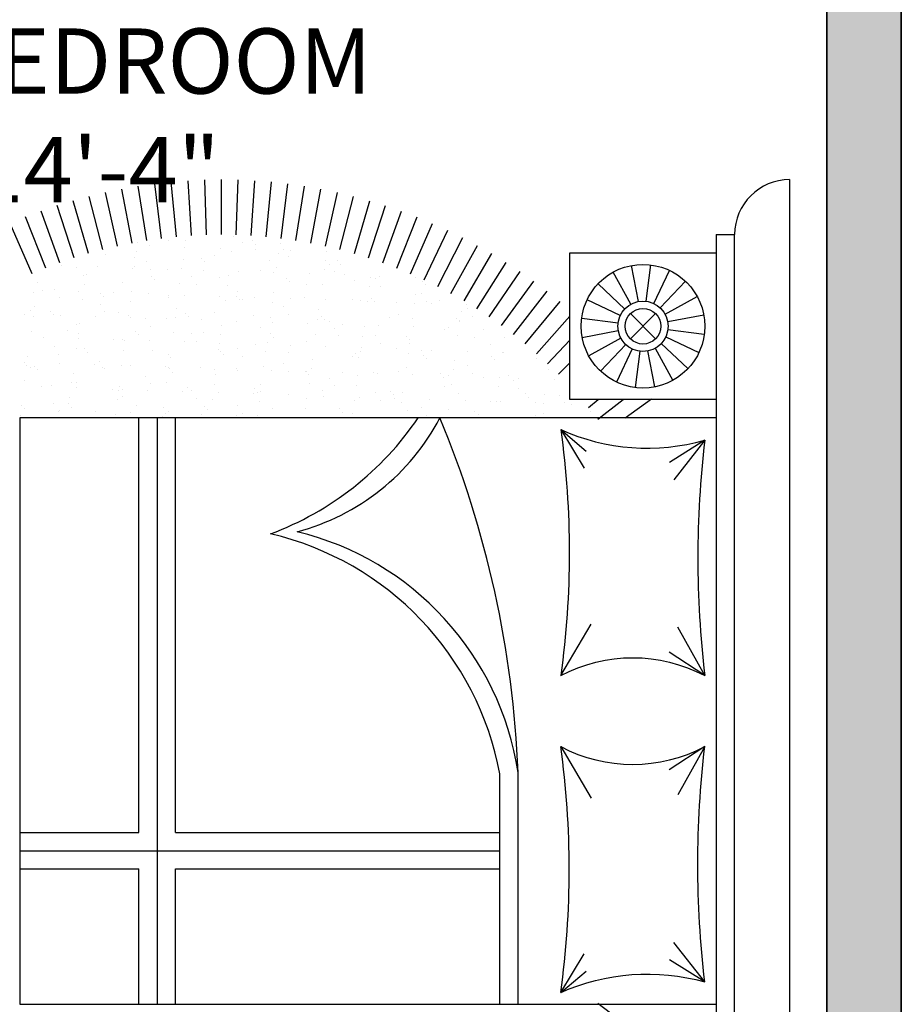
# Model space of a CAD drawing. Units: inches. Extents: x 1566 to 2546, y 1087 to 2705.
# Tile 17 of 27: x 2364 to 2458, y 1243 to 1349. Entities that reach past the tile are written whole.
import ezdxf

# ---------------------------------------------------------------- set-up
doc = ezdxf.new("R2010")
doc.units = ezdxf.units.IN
for name, color, linetype, lineweight in [('A-AREA-IDEN', 7, 'Continuous', 18), ('A-FURN', 8, 'Continuous', 18), ('A-WALL', 7, 'Continuous', 35), ('A-WALL-PATT', 8, 'Continuous', 13)]:
    doc.layers.add(name, color=color, linetype=linetype, lineweight=lineweight)
for name, color, linetype in [('A-FRN', 11, 'Continuous'), ('A-HT', 15, 'Continuous'), ('L-HT', 1, 'Continuous')]:
    doc.layers.add(name, color=color, linetype=linetype)
doc.styles.get("Standard").update_dxf_attribs({"font": 'arial.ttf'})

# ---------------------------------------------------------------- blocks, each defined once
blk = doc.blocks.new('*X21')
at = {"color": 0}
for p, q in [((1.1667, 2.0955), (1.1667, 2.0955)), ((1.1927, 2.0989), (1.1927, 2.0989)), ((0.9061, 2.0695), (0.9061, 2.0695)), ((0.9169, 2.0861), (0.9169, 2.0861)), ((0.9642, 2.0688), (0.9642, 2.0688)), ((1.0321, 2.0777), (1.0321, 2.0777)), ((1.0477, 2.0878), (1.0477, 2.0878)), ((1.0582, 2.0812), (1.0582, 2.0812)), ((1.0618, 2.0698), (1.0618, 2.0698)), ((1.0988, 2.0865), (1.0988, 2.0865)), ((1.1756, 2.0872), (1.1756, 2.0872)), ((0.8296, 2.0511), (0.8296, 2.0511)), ((0.8589, 2.0624), (0.8589, 2.0624)), ((0.8975, 2.06), (0.8975, 2.06)), ((0.9236, 2.0635), (0.9236, 2.0635)), ((1.059, 2.0607), (1.059, 2.0607)), ((1.0682, 2.0523), (1.0682, 2.0523)), ((0.8524, 2.0367), (0.8524, 2.0367)), ((0.9087, 2.0168), (0.9087, 2.0168)), ((0.9803, 2.0361), (0.9803, 2.0361)), ((1.1153, 2.0409), (1.1153, 2.0409)), ((0.8495, 2.0061), (0.8495, 2.0061)), ((0.8706, 1.9927), (0.8706, 1.9927)), ((0.9179, 2.0084), (0.9179, 2.0084)), ((0.92, 1.9898), (0.92, 1.9898)), ((1.0052, 2.0064), (1.0052, 2.0064)), ((1.0263, 1.993), (1.0263, 1.993)), ((1.0509, 1.9915), (1.0509, 1.9915)), ((1.1117, 2.0124), (1.1117, 2.0124)), ((1.1609, 2.0067), (1.1609, 2.0067)), ((1.1788, 1.9909), (1.1788, 1.9909)), ((1.182, 1.9932), (1.182, 1.9932)), ((0.785, 1.9849), (0.785, 1.9849)), ((0.9614, 1.9685), (0.9614, 1.9685)), ((1.1449, 1.9631), (1.1449, 1.9631)), ((1.1614, 1.9668), (1.1614, 1.9668)), ((0.7908, 1.944), (0.7908, 1.944)), ((0.8555, 1.9403), (0.8555, 1.9403)), ((0.9436, 1.9366), (0.9436, 1.9366)), ((0.9465, 1.9443), (0.9465, 1.9443)), ((0.9697, 1.9401), (0.9697, 1.9401)), ((0.9834, 1.9397), (0.9834, 1.9397)), ((1.0103, 1.9454), (1.0103, 1.9454)), ((1.0782, 1.9544), (1.0782, 1.9544)), ((1.1022, 1.9446), (1.1022, 1.9446)), ((1.1043, 1.9578), (1.1043, 1.9578)), ((1.1185, 1.9446), (1.1185, 1.9446)), ((1.1707, 1.9584), (1.1707, 1.9584)), ((0.8091, 1.9189), (0.8091, 1.9189)), ((0.8111, 1.9247), (0.8111, 1.9247)), ((0.8351, 1.9223), (0.8351, 1.9223)), ((0.8757, 1.9277), (0.8757, 1.9277)), ((1.0111, 1.9229), (1.0111, 1.9229)), ((1.0204, 1.9145), (1.0204, 1.9145)), ((0.7881, 1.8886), (0.7881, 1.8886)), ((0.8898, 1.8809), (0.8898, 1.8809)), ((0.9232, 1.8935), (0.9232, 1.8935)), ((1.0456, 1.8812), (1.0456, 1.8812)), ((1.054, 1.8951), (1.054, 1.8951)), ((1.1819, 1.8945), (1.1819, 1.8945)), ((0.7552, 1.8672), (0.7552, 1.8672)), ((0.8608, 1.879), (0.8608, 1.879)), ((0.8701, 1.8706), (0.8701, 1.8706)), ((0.9109, 1.8675), (0.9109, 1.8675)), ((1.0639, 1.8746), (1.0639, 1.8746)), ((1.0666, 1.8678), (1.0666, 1.8678)), ((0.8587, 1.844), (0.8587, 1.844)), ((0.9136, 1.8307), (0.9136, 1.8307)), ((0.9866, 1.8434), (0.9866, 1.8434)), ((1.1136, 1.829), (1.1136, 1.829)), ((1.1216, 1.8482), (1.1216, 1.8482)), ((1.1243, 1.831), (1.1243, 1.831)), ((1.1504, 1.8344), (1.1504, 1.8344)), ((1.191, 1.8397), (1.191, 1.8397)), ((0.8311, 1.8188), (0.8311, 1.8188)), ((0.9218, 1.8043), (0.9218, 1.8043)), ((0.9868, 1.8191), (0.9868, 1.8191)), ((0.9897, 1.8132), (0.9897, 1.8132)), ((1.0158, 1.8167), (1.0158, 1.8167)), ((1.0564, 1.822), (1.0564, 1.822)), ((1.1228, 1.8206), (1.1228, 1.8206)), ((1.1425, 1.8194), (1.1425, 1.8194)), ((0.7206, 1.7778), (0.7206, 1.7778)), ((0.7466, 1.7812), (0.7466, 1.7812)), ((0.7632, 1.7869), (0.7632, 1.7869)), ((0.7872, 1.7866), (0.7872, 1.7866)), ((0.7913, 1.7922), (0.7913, 1.7922)), ((0.8552, 1.7955), (0.8552, 1.7955)), ((0.8812, 1.799), (0.8812, 1.799)), ((0.9263, 1.7971), (0.9263, 1.7971)), ((0.9633, 1.7851), (0.9633, 1.7851)), ((0.9725, 1.7767), (0.9725, 1.7767)), ((1.0572, 1.7988), (1.0572, 1.7988)), ((1.1663, 1.7807), (1.1663, 1.7807)), ((1.1851, 1.7982), (1.1851, 1.7982)), ((0.7745, 1.7554), (0.7745, 1.7554)), ((0.8618, 1.7477), (0.8618, 1.7477)), ((0.9302, 1.7557), (0.9302, 1.7557)), ((0.9897, 1.747), (0.9897, 1.747)), ((1.0859, 1.756), (1.0859, 1.756)), ((1.1248, 1.7519), (1.1248, 1.7519)), ((0.731, 1.746), (0.731, 1.746)), ((0.7956, 1.742), (0.7956, 1.742)), ((0.813, 1.7413), (0.813, 1.7413)), ((0.8222, 1.7328), (0.8222, 1.7328)), ((0.9513, 1.7423), (0.9513, 1.7423)), ((1.016, 1.7368), (1.016, 1.7368)), ((1.107, 1.7426), (1.107, 1.7426)), ((0.7158, 1.6933), (0.7158, 1.6933)), ((0.7944, 1.6959), (0.7944, 1.6959)), ((0.8657, 1.693), (0.8657, 1.693)), ((0.8715, 1.6936), (0.8715, 1.6936)), ((0.9295, 1.7008), (0.9295, 1.7008)), ((1.0272, 1.6939), (1.0272, 1.6939)), ((1.0603, 1.7024), (1.0603, 1.7024)), ((1.0619, 1.6933), (1.0619, 1.6933)), ((1.1025, 1.6986), (1.1025, 1.6986)), ((1.1704, 1.7076), (1.1704, 1.7076)), ((1.1829, 1.6942), (1.1829, 1.6942)), ((1.1882, 1.7018), (1.1882, 1.7018)), ((1.1965, 1.711), (1.1965, 1.711)), ((0.9013, 1.6721), (0.9013, 1.6721)), ((0.9273, 1.6756), (0.9273, 1.6756)), ((0.9679, 1.6809), (0.9679, 1.6809)), ((1.0358, 1.6899), (1.0358, 1.6899)), ((1.0658, 1.6912), (1.0658, 1.6912)), ((1.075, 1.6828), (1.075, 1.6828)), ((0.7154, 1.6491), (0.7154, 1.6491)), ((0.7341, 1.6496), (0.7341, 1.6496)), ((0.7667, 1.6544), (0.7667, 1.6544)), ((0.7927, 1.6578), (0.7927, 1.6578)), ((0.8333, 1.6632), (0.8333, 1.6632)), ((0.865, 1.6513), (0.865, 1.6513)), ((0.9155, 1.6474), (0.9155, 1.6474)), ((0.9247, 1.6389), (0.9247, 1.6389)), ((0.9929, 1.6507), (0.9929, 1.6507)), ((1.1185, 1.6429), (1.1185, 1.6429)), ((1.1279, 1.6556), (1.1279, 1.6556)), ((0.8149, 1.6302), (0.8149, 1.6302)), ((0.836, 1.6168), (0.836, 1.6168)), ((0.9706, 1.6305), (0.9706, 1.6305)), ((0.9917, 1.6171), (0.9917, 1.6171)), ((1.1263, 1.6308), (1.1263, 1.6308)), ((1.1474, 1.6173), (1.1474, 1.6173)), ((0.7652, 1.6035), (0.7652, 1.6035)), ((0.7744, 1.595), (0.7744, 1.595)), ((0.7976, 1.5996), (0.7976, 1.5996)), ((0.9326, 1.6044), (0.9326, 1.6044)), ((0.9682, 1.599), (0.9682, 1.599)), ((1.0635, 1.6061), (1.0635, 1.6061)), ((1.1683, 1.5973), (1.1683, 1.5973)), ((1.1775, 1.5889), (1.1775, 1.5889)), ((1.1914, 1.6055), (1.1914, 1.6055)), ((0.7562, 1.5681), (0.7562, 1.5681)), ((0.9119, 1.5684), (0.9119, 1.5684)), ((1.0676, 1.5687), (1.0676, 1.5687)), ((1.0819, 1.5665), (1.0819, 1.5665)), ((1.108, 1.5699), (1.108, 1.5699)), ((1.1311, 1.5592), (1.1311, 1.5592)), ((1.1486, 1.5753), (1.1486, 1.5753)), ((0.7373, 1.5533), (0.7373, 1.5533)), ((0.8179, 1.5552), (0.8179, 1.5552)), ((0.8388, 1.5345), (0.8388, 1.5345)), ((0.8681, 1.555), (0.8681, 1.555)), ((0.8794, 1.5398), (0.8794, 1.5398)), ((0.9474, 1.5488), (0.9474, 1.5488)), ((0.9734, 1.5522), (0.9734, 1.5522)), ((0.996, 1.5544), (0.996, 1.5544)), ((1.014, 1.5575), (1.014, 1.5575)), ((1.018, 1.5534), (1.018, 1.5534)), ((1.0272, 1.545), (1.0272, 1.545)), ((0.7042, 1.5167), (0.7042, 1.5167)), ((0.7448, 1.5221), (0.7448, 1.5221)), ((0.8128, 1.531), (0.8128, 1.531)), ((0.8553, 1.505), (0.8553, 1.505)), ((0.8677, 1.5096), (0.8677, 1.5096)), ((0.9358, 1.5081), (0.9358, 1.5081)), ((1.011, 1.5053), (1.011, 1.5053)), ((1.0666, 1.5098), (1.0666, 1.5098)), ((1.0707, 1.5051), (1.0707, 1.5051)), ((1.1667, 1.5056), (1.1667, 1.5056)), ((1.1945, 1.5091), (1.1945, 1.5091)), ((0.7207, 1.4913), (0.7207, 1.4913)), ((0.8007, 1.5032), (0.8007, 1.5032)), ((0.8764, 1.4916), (0.8764, 1.4916)), ((0.8769, 1.5011), (0.8769, 1.5011)), ((1.0321, 1.4919), (1.0321, 1.4919)), ((1.1878, 1.4921), (1.1878, 1.4921)), ((0.7174, 1.4657), (0.7174, 1.4657)), ((0.7266, 1.4572), (0.7266, 1.4572)), ((0.7404, 1.457), (0.7404, 1.457)), ((0.8713, 1.4586), (0.8713, 1.4586)), ((0.9204, 1.4613), (0.9204, 1.4613)), ((0.9992, 1.458), (0.9992, 1.458)), ((1.1205, 1.4595), (1.1205, 1.4595)), ((1.1297, 1.4511), (1.1297, 1.4511)), ((1.1342, 1.4629), (1.1342, 1.4629)), ((1.1947, 1.4519), (1.1947, 1.4519)), ((0.7966, 1.4429), (0.7966, 1.4429)), ((0.9523, 1.4432), (0.9523, 1.4432)), ((0.9935, 1.4254), (0.9935, 1.4254)), ((1.0195, 1.4288), (1.0195, 1.4288)), ((1.0601, 1.4341), (1.0601, 1.4341)), ((1.108, 1.4435), (1.108, 1.4435)), ((1.128, 1.4431), (1.128, 1.4431)), ((1.1541, 1.4465), (1.1541, 1.4465)), ((0.7701, 1.4174), (0.7701, 1.4174)), ((0.7909, 1.3987), (0.7909, 1.3987)), ((0.8039, 1.4069), (0.8039, 1.4069)), ((0.8589, 1.4076), (0.8589, 1.4076)), ((0.8849, 1.4111), (0.8849, 1.4111)), ((0.9255, 1.4164), (0.9255, 1.4164)), ((0.9389, 1.4118), (0.9389, 1.4118)), ((0.9701, 1.4157), (0.9701, 1.4157)), ((0.9794, 1.4072), (0.9794, 1.4072)), ((1.0698, 1.4134), (1.0698, 1.4134)), ((1.1732, 1.4112), (1.1732, 1.4112)), ((1.1977, 1.4128), (1.1977, 1.4128)), ((0.7243, 1.3899), (0.7243, 1.3899)), ((0.74, 1.3795), (0.74, 1.3795)), ((0.7503, 1.3934), (0.7503, 1.3934)), ((0.8198, 1.3718), (0.8198, 1.3718)), ((0.8957, 1.3798), (0.8957, 1.3798)), ((1.0514, 1.3801), (1.0514, 1.3801)), ((0.7436, 1.3606), (0.7436, 1.3606)), ((0.761, 1.3661), (0.761, 1.3661)), ((0.8291, 1.3633), (0.8291, 1.3633)), ((0.8744, 1.3623), (0.8744, 1.3623)), ((0.9168, 1.3664), (0.9168, 1.3664)), ((1.0023, 1.3617), (1.0023, 1.3617)), ((1.0229, 1.3673), (1.0229, 1.3673)), ((1.0725, 1.3667), (1.0725, 1.3667)), ((1.1374, 1.3665), (1.1374, 1.3665)), ((0.837, 1.3177), (0.837, 1.3177)), ((0.8726, 1.3235), (0.8726, 1.3235)), ((0.9927, 1.318), (0.9927, 1.318)), ((1.0726, 1.3217), (1.0726, 1.3217)), ((1.0729, 1.3171), (1.0729, 1.3171)), ((1.1484, 1.3183), (1.1484, 1.3183)), ((1.1741, 1.3197), (1.1741, 1.3197)), ((0.807, 1.3105), (0.807, 1.3105)), ((0.9421, 1.3154), (0.9421, 1.3154)), ((0.9716, 1.293), (0.9716, 1.293)), ((1.0396, 1.302), (1.0396, 1.302)), ((1.0656, 1.3054), (1.0656, 1.3054)), ((1.0818, 1.3133), (1.0818, 1.3133)), ((1.1062, 1.3108), (1.1062, 1.3108)), ((0.7467, 1.2643), (0.7467, 1.2643)), ((0.7704, 1.2665), (0.7704, 1.2665)), ((0.7964, 1.27), (0.7964, 1.27)), ((0.837, 1.2753), (0.837, 1.2753)), ((0.8776, 1.2659), (0.8776, 1.2659)), ((0.905, 1.2843), (0.905, 1.2843)), ((0.9223, 1.2779), (0.9223, 1.2779)), ((0.931, 1.2877), (0.931, 1.2877)), ((0.9315, 1.2694), (0.9315, 1.2694)), ((1.0055, 1.2653), (1.0055, 1.2653)), ((1.1253, 1.2734), (1.1253, 1.2734)), ((1.1405, 1.2702), (1.1405, 1.2702)), ((0.7803, 1.2543), (0.7803, 1.2543)), ((0.8014, 1.2409), (0.8014, 1.2409)), ((0.936, 1.2546), (0.936, 1.2546)), ((0.9571, 1.2412), (0.9571, 1.2412)), ((1.0918, 1.2549), (1.0918, 1.2549)), ((1.1128, 1.2414), (1.1128, 1.2414)), ((0.772, 1.234), (0.772, 1.234)), ((0.7812, 1.2255), (0.7812, 1.2255)), ((0.8102, 1.2142), (0.8102, 1.2142)), ((0.9452, 1.2191), (0.9452, 1.2191)), ((0.975, 1.2296), (0.975, 1.2296)), ((1.0761, 1.2207), (1.0761, 1.2207)), ((1.1751, 1.2278), (1.1751, 1.2278)), ((1.1843, 1.2194), (1.1843, 1.2194)), ((0.8247, 1.1857), (0.8247, 1.1857)), ((0.8773, 1.1925), (0.8773, 1.1925)), ((1.0248, 1.184), (1.0248, 1.184)), ((1.033, 1.1928), (1.033, 1.1928)), ((1.1523, 1.1874), (1.1523, 1.1874)), ((1.1887, 1.1931), (1.1887, 1.1931)), ((0.8807, 1.1696), (0.8807, 1.1696)), ((0.9511, 1.1609), (0.9511, 1.1609)), ((0.9771, 1.1643), (0.9771, 1.1643)), ((1.0086, 1.169), (1.0086, 1.169)), ((1.0177, 1.1696), (1.0177, 1.1696)), ((1.034, 1.1755), (1.034, 1.1755)), ((1.0857, 1.1786), (1.0857, 1.1786)), ((1.1117, 1.182), (1.1117, 1.182)), ((1.1437, 1.1739), (1.1437, 1.1739)), ((0.8165, 1.1432), (0.8165, 1.1432)), ((0.8207, 1.1291), (0.8207, 1.1291)), ((0.8425, 1.1466), (0.8425, 1.1466)), ((0.8745, 1.1401), (0.8745, 1.1401)), ((0.8831, 1.1519), (0.8831, 1.1519)), ((0.8837, 1.1316), (0.8837, 1.1316)), ((0.9764, 1.1294), (0.9764, 1.1294)), ((1.0775, 1.1356), (1.0775, 1.1356)), ((1.1321, 1.1297), (1.1321, 1.1297)), ((0.8133, 1.1179), (0.8133, 1.1179)), ((0.8418, 1.1157), (0.8418, 1.1157)), ((0.9484, 1.1227), (0.9484, 1.1227)), ((0.9975, 1.116), (0.9975, 1.116)), ((1.0792, 1.1244), (1.0792, 1.1244)), ((1.1532, 1.1162), (1.1532, 1.1162)), ((0.9272, 1.0918), (0.9272, 1.0918)), ((1.1273, 1.09), (1.1273, 1.09)), ((1.1365, 1.0816), (1.1365, 1.0816)), ((1.1468, 1.0775), (1.1468, 1.0775)), ((0.8839, 1.0733), (0.8839, 1.0733)), ((0.9177, 1.0673), (0.9177, 1.0673)), ((1.0118, 1.0727), (1.0118, 1.0727)), ((1.0734, 1.0676), (1.0734, 1.0676)), ((1.1318, 1.0552), (1.1318, 1.0552)), ((1.1578, 1.0586), (1.1578, 1.0586)), ((1.1984, 1.064), (1.1984, 1.064)), ((0.8165, 1.0215), (0.8165, 1.0215)), ((0.8886, 1.0232), (0.8886, 1.0232)), ((0.9292, 1.0285), (0.9292, 1.0285)), ((0.9515, 1.0264), (0.9515, 1.0264)), ((0.977, 1.0462), (0.977, 1.0462)), ((0.9862, 1.0377), (0.9862, 1.0377)), ((0.9972, 1.0375), (0.9972, 1.0375)), ((1.0232, 1.0409), (1.0232, 1.0409)), ((1.0638, 1.0463), (1.0638, 1.0463)), ((1.0824, 1.0281), (1.0824, 1.0281)), ((1.18, 1.0417), (1.18, 1.0417)), ((0.8267, 1.0023), (0.8267, 1.0023)), ((0.8611, 1.0039), (0.8611, 1.0039)), ((0.8626, 1.0198), (0.8626, 1.0198)), ((1.0168, 1.0042), (1.0168, 1.0042)), ((1.0297, 0.9979), (1.0297, 0.9979)), ((1.1725, 1.0045), (1.1725, 1.0045)), ((0.8359, 0.9938), (0.8359, 0.9938)), ((0.8822, 0.9905), (0.8822, 0.9905)), ((0.887, 0.9769), (0.887, 0.9769)), ((1.0149, 0.9763), (1.0149, 0.9763)), ((1.0379, 0.9908), (1.0379, 0.9908)), ((1.15, 0.9812), (1.15, 0.9812)), ((1.1936, 0.991), (1.1936, 0.991)), ((0.8794, 0.954), (0.8794, 0.954)), ((0.9581, 0.9421), (0.9581, 0.9421)), ((1.0795, 0.9523), (1.0795, 0.9523)), ((1.0887, 0.9438), (1.0887, 0.9438)), ((1.1138, 0.9424), (1.1138, 0.9424)), ((0.9546, 0.93), (0.9546, 0.93)), ((1.0433, 0.9141), (1.0433, 0.9141)), ((1.0693, 0.9175), (1.0693, 0.9175)), ((1.0855, 0.9317), (1.0855, 0.9317)), ((1.1099, 0.9229), (1.1099, 0.9229)), ((1.1779, 0.9318), (1.1779, 0.9318)), ((0.9087, 0.8964), (0.9087, 0.8964)), ((0.9292, 0.9084), (0.9292, 0.9084)), ((0.9347, 0.8998), (0.9347, 0.8998)), ((0.9384, 0.8999), (0.9384, 0.8999)), ((0.9753, 0.9052), (0.9753, 0.9052)), ((1.1322, 0.904), (1.1322, 0.904)), ((0.8902, 0.8806), (0.8902, 0.8806)), ((0.9015, 0.8787), (0.9015, 0.8787)), ((0.9226, 0.8653), (0.9226, 0.8653)), ((0.9819, 0.8601), (0.9819, 0.8601)), ((1.0181, 0.88), (1.0181, 0.88)), ((1.0572, 0.879), (1.0572, 0.879)), ((1.0783, 0.8655), (1.0783, 0.8655)), ((1.1531, 0.8848), (1.1531, 0.8848)), ((0.9578, 0.8337), (0.9578, 0.8337)), ((1.0887, 0.8354), (1.0887, 0.8354)), ((1.1819, 0.8583), (1.1819, 0.8583)), ((1.1912, 0.8499), (1.1912, 0.8499)), ((0.9985, 0.8169), (0.9985, 0.8169)), ((1.0316, 0.8145), (1.0316, 0.8145)), ((1.0409, 0.806), (1.0409, 0.806)), ((1.1542, 0.8172), (1.1542, 0.8172)), ((1.0212, 0.7836), (1.0212, 0.7836)), ((1.0214, 0.7818), (1.0214, 0.7818)), ((1.0894, 0.7907), (1.0894, 0.7907)), ((1.1154, 0.7941), (1.1154, 0.7941)), ((1.156, 0.7995), (1.156, 0.7995)), ((1.1563, 0.7885), (1.1563, 0.7885)), ((0.9808, 0.7764), (0.9808, 0.7764)), ((1.0844, 0.7662), (1.0844, 0.7662)), ((1.0976, 0.7538), (1.0976, 0.7538)), ((1.0918, 0.739), (1.0918, 0.739)), ((1.1187, 0.7403), (1.1187, 0.7403)), ((1.1341, 0.7206), (1.1341, 0.7206)), ((1.1433, 0.7121), (1.1433, 0.7121)), ((1.0389, 0.6917), (1.0389, 0.6917)), ((1.1594, 0.6922), (1.1594, 0.6922)), ((1.1868, 0.6723), (1.1868, 0.6723)), ((1.1946, 0.692), (1.1946, 0.692)), ((1.0675, 0.6584), (1.0675, 0.6584)), ((1.1355, 0.6673), (1.1355, 0.6673)), ((1.1615, 0.6707), (1.1615, 0.6707)), ((1.095, 0.6427), (1.095, 0.6427)), ((1.138, 0.6286), (1.138, 0.6286)), ((1.159, 0.6151), (1.159, 0.6151)), ((1.1626, 0.5958), (1.1626, 0.5958)), ((1.1816, 0.5439), (1.1816, 0.5439))]:
    blk.add_line(p, q, dxfattribs=at)
blk = doc.blocks.new('A$C6796526C')
at = {"layer": 'A-FRN'}
for p, q in [((0, 3), (2.9, 3)), ((2.75, 2.85), (0.15, 2.85)), ((0.15, 2.8), (0.15, 2.85)), ((0.15, 2.8), (2.75, 2.8)), ((0.2, 2.4), (0.2, 2.8)), ((0.6, 2.8), (0.6, 2.4)), ((0.6, 2.4), (0.2, 2.4))]:
    blk.add_line(p, q, dxfattribs=at)
blk.add_lwpolyline([(0.65, 2.8), (0.65, 0.9), (2.25, 0.9), (2.25, 2.8)], dxfattribs=at)
for points in [[(0.6821, 2.3755, 0.175461), (0.7109, 2.7686)], [(0.7109, 2.7686, 0.059544), (1.3533, 2.7686)], [(1.3533, 2.3755, -0.248743), (1.3533, 2.7686)], [(2.1891, 2.7686, -0.059544), (1.5467, 2.7686)], [(1.5467, 2.3755, 0.248743), (1.5467, 2.7686)], [(2.2179, 2.3755, -0.175461), (2.1891, 2.7686)], [(0.6821, 2.3755, -0.069628), (1.3533, 2.3755)], [(2.2179, 2.3755, 0.069628), (1.5467, 2.3755)], [(2.25, 2.2594), (1.6173, 2.2594, 0.303651), (0.9607, 1.6568, 0.210515), (0.65, 2.0462)]]:
    blk.add_lwpolyline(points, format="xyb", dxfattribs=at)
for radius in [0.1686, 0.0686]:
    blk.add_circle((0.4, 2.6), radius, dxfattribs=at)
for centre, radius, start, end in [((0.15, 3), 0.15, 180, 270), ((1.7313, -0.5592), 2.8209, 92.3174, 112.5397)]:
    blk.add_arc(centre, radius, start, end, dxfattribs=at)
at = {"layer": 'A-HT'}
for p, q in [((0.65, 2.5511), (0.5977, 2.6231)), ((0.6532, 2.4772), (0.6, 2.5458)), ((2.2468, 2.4772), (2.3, 2.5458)), ((0.6213, 2.4517), (0.6, 2.4775)), ((0.4749, 2.3097), (0.3724, 2.4)), ((0.5023, 2.3399), (0.4384, 2.4)), ((0.5308, 2.3692), (0.5, 2.4)), ((0.4483, 2.2787), (0.3328, 2.3743)), ((0.4228, 2.2468), (0.3043, 2.3387)), ((0.3983, 2.2141), (0.2769, 2.3023)), ((0.3748, 2.1807), (0.2507, 2.265)), ((0.3524, 2.1466), (0.2257, 2.2269)), ((0.331, 2.1118), (0.2019, 2.1881)), ((0.3108, 2.0763), (0.1794, 2.1485)), ((0.2917, 2.0402), (0.158, 2.1083)), ((0.2737, 2.0035), (0.138, 2.0674)), ((0.2569, 1.9663), (0.1193, 2.0259)), ((0.2413, 1.9286), (0.1018, 1.9838)), ((0.2269, 1.8904), (0.0857, 1.9412)), ((0.2136, 1.8517), (0.071, 1.8981)), ((0.2016, 1.8127), (0.0576, 1.8545)), ((0.1908, 1.7733), (0.0456, 1.8106)), ((0.1813, 1.7336), (0.0349, 1.7663)), ((0.173, 1.6936), (0.0257, 1.7217)), ((0.166, 1.6534), (0.0179, 1.6768)), ((0.1603, 1.6129), (0.0114, 1.6317)), ((0.1558, 1.5723), (0.0064, 1.5865)), ((0.1526, 1.5316), (0.0029, 1.541)), ((0.1506, 1.4908), (0.0007, 1.4955)), ((0.15, 1.45), (0, 1.45)), ((0.1506, 1.4092), (0.0007, 1.4045)), ((0.1526, 1.3684), (0.0029, 1.359)), ((0.1558, 1.3277), (0.0064, 1.3135)), ((0.1603, 1.2871), (0.0114, 1.2683)), ((0.166, 1.2466), (0.0179, 1.2232)), ((0.173, 1.2064), (0.0257, 1.1783)), ((0.1813, 1.1664), (0.0349, 1.1337)), ((0.1908, 1.1267), (0.0456, 1.0894)), ((0.2016, 1.0873), (0.0576, 1.0455)), ((0.2136, 1.0483), (0.071, 1.0019)), ((0.2269, 1.0096), (0.0857, 0.9588)), ((0.2413, 0.9714), (0.1018, 0.9162)), ((0.2569, 0.9337), (0.1193, 0.8741))]:
    blk.add_line(p, q, dxfattribs=at)
at = {"layer": 'L-HT'}
for p, q in [((0.4087, 2.668), (0.4214, 2.7672)), ((0.7109, 2.7686), (0.8188, 2.6839)), ((0.7109, 2.7686), (0.7717, 2.6727)), ((1.3533, 2.7686), (1.2212, 2.6952)), ((1.3533, 2.7686), (1.2893, 2.6715)), ((1.5467, 2.7686), (1.6107, 2.6715)), ((1.5467, 2.7686), (1.6788, 2.6952)), ((2.1891, 2.7686), (2.0812, 2.6839)), ((2.1891, 2.7686), (2.1283, 2.6727)), ((0.3671, 2.6601), (0.319, 2.7478)), ((0.3873, 2.6674), (0.3687, 2.7656)), ((0.4293, 2.662), (0.472, 2.7524)), ((0.3501, 2.647), (0.2773, 2.7156)), ((0.447, 2.6499), (0.5156, 2.7227)), ((0.338, 2.6293), (0.2476, 2.672)), ((0.4601, 2.6329), (0.5478, 2.681)), ((0.3657, 2.5657), (0.4343, 2.6343)), ((0.4343, 2.5657), (0.3657, 2.6343)), ((0.332, 2.6087), (0.2328, 2.6214)), ((0.4674, 2.6127), (0.5656, 2.6313)), ((0.3326, 2.5873), (0.2344, 2.5687)), ((0.468, 2.5913), (0.5672, 2.5786)), ((0.3399, 2.5671), (0.2522, 2.519)), ((0.4499, 2.553), (0.5227, 2.4844)), ((0.462, 2.5707), (0.5524, 2.528)), ((0.353, 2.5501), (0.2844, 2.4773)), ((0.3707, 2.538), (0.328, 2.4476)), ((0.3913, 2.532), (0.3786, 2.4328)), ((0.4127, 2.5326), (0.4313, 2.4344)), ((0.4329, 2.5399), (0.481, 2.4522)), ((1.3533, 2.3755), (1.2125, 2.4585)), ((1.5467, 2.3755), (1.6875, 2.4585)), ((0.6821, 2.3755), (0.7405, 2.4447)), ((0.6821, 2.3755), (0.7872, 2.4395)), ((2.2179, 2.3755), (2.1128, 2.4395)), ((2.2179, 2.3755), (2.1595, 2.4447)), ((2.25, 2.2094), (1.6212, 2.2094)), ((1.7809, 1.3249), (1.7809, 2.2094)), ((1.8309, 0.9), (1.8309, 2.2094)), ((1.8809, 1.3249), (1.8809, 2.2094)), ((1.7809, 1.3249), (0.65, 1.3249)), ((2.25, 1.3249), (1.8809, 1.3249)), ((0.65, 1.2749), (2.25, 1.2749)), ((1.7809, 1.2249), (0.65, 1.2249)), ((1.7809, 0.9), (1.7809, 1.2249)), ((1.8809, 0.9), (1.8809, 1.2249)), ((2.25, 1.2249), (1.8809, 1.2249))]:
    blk.add_line(p, q, dxfattribs=at)
blk.add_circle((0.4, 2.6), 0.0486, dxfattribs=at)
for centre, radius, start, end in [((1.7721, 1.396), 0.8272, 100.5107, 166.872), ((0.1786, 1.2908), 0.8406, 20.4105, 55.8901)]:
    blk.add_arc(centre, radius, start, end, dxfattribs=at)
at = {"layer": 'A-HT', "extrusion": (0, 0, -1), "zscale": -1, "rotation": 180}
blk.add_blockref('*X21', (0.55, 3), dxfattribs=at)

msp = doc.modelspace()

# ---------------------------------------------------------------- hatches: boundary and pattern name
at = {"layer": 'A-WALL-PATT'}
h = msp.add_hatch(color=256, dxfattribs=at)
h.dxf.hatch_style = 1
h.paths.add_polyline_path([(2106.29, 1385.43), (2228.29, 1385.43), (2228.29, 1391.43), (2224.29, 1391.43), (2224.29, 1389.43), (2106.29, 1389.43), (2106.29, 1402.93), (2098.29, 1402.93), (2098.29, 1343.43), (2106.29, 1343.43), (2106.29, 1347.74)], flags=17)
h.paths.add_polyline_path([(2106.29, 1259.43), (2098.29, 1259.43), (2098.29, 1209.43), (2155.29, 1209.43), (2155.29, 1217.43), (2143.41, 1217.43), (2106.29, 1217.43)], flags=17)
h.paths.add_polyline_path([(2334.29, 1217.43), (2280.29, 1217.43), (2280.29, 1389.43), (2284.29, 1389.43), (2284.29, 1391.43), (2284.29, 1393.43), (2276.29, 1393.43), (2276.29, 1217.43), (2227.29, 1217.43), (2227.29, 1209.43), (2334.29, 1209.43)], flags=17)
h.paths.add_polyline_path([(2106.29, 1486.43), (2098.29, 1486.43), (2098.29, 1460.88), (2099.11, 1461.64), (2100.44, 1462.65), (2101.57, 1463.26), (2099.97, 1460.62), (2098.29, 1458.1), (2098.29, 1456.93), (2100.35, 1456.93), (2100.77, 1457.12), (2103.56, 1457.95), (2106.29, 1458.4), (2106.29, 1470.43), (2224.29, 1470.43), (2224.29, 1427.43), (2228.29, 1427.43), (2228.29, 1474.43), (2192.29, 1474.43), (2192.29, 1476.43), (2188.29, 1476.43), (2188.29, 1474.43), (2106.29, 1474.43)], flags=17)
h.paths.add_polyline_path([(2106.29, 1585.43), (2192.29, 1585.43), (2192.29, 1589.43), (2098.29, 1589.43), (2098.29, 1573.93), (2106.29, 1573.93)], flags=17)
h.paths.add_polyline_path([(2228.29, 1585.43), (2232.29, 1585.43), (2232.29, 1589.43), (2224.29, 1589.43), (2222.29, 1589.43), (2222.29, 1585.43), (2224.29, 1585.43), (2224.29, 1532.43), (2106.29, 1532.43), (2106.29, 1543.93), (2098.29, 1543.93), (2098.29, 1516.43), (2106.29, 1516.43), (2106.29, 1528.43), (2188.29, 1528.43), (2188.29, 1506.43), (2192.29, 1506.43), (2192.29, 1528.43), (2224.29, 1528.43), (2224.29, 1506.43), (2228.29, 1506.43)], flags=17)
h.paths.add_polyline_path([(2106.29, 1680.43), (2098.29, 1680.43), (2098.29, 1625.43), (2106.29, 1625.43)], flags=17)
h.paths.add_polyline_path([(2458.29, 1784.43), (2098.29, 1784.43), (2098.29, 1776.43), (2276.29, 1776.43), (2276.29, 1589.43), (2268.29, 1589.43), (2268.29, 1585.43), (2280.29, 1585.43), (2280.29, 1652.43), (2284.29, 1652.43), (2284.29, 1656.43), (2280.29, 1656.43), (2280.29, 1776.43), (2398.29, 1776.43), (2398.29, 1746.43), (2402.29, 1746.43), (2402.29, 1776.43), (2450.29, 1776.43), (2450.29, 1532.43), (2375.49, 1532.43), (2328.29, 1532.43), (2328.29, 1612.43), (2324.29, 1612.43), (2324.29, 1528.43), (2450.29, 1528.43), (2450.29, 1447.43), (2291.29, 1447.43), (2291.29, 1443.43), (2324.29, 1443.43), (2324.29, 1393.43), (2320.29, 1393.43), (2320.29, 1389.43), (2330.29, 1389.43), (2330.29, 1393.43), (2328.29, 1393.43), (2328.29, 1443.43), (2412.29, 1443.43), (2412.29, 1433.43), (2416.29, 1433.43), (2416.29, 1443.43), (2450.29, 1443.43), (2450.29, 1393.43), (2416.29, 1393.43), (2416.29, 1403.43), (2412.29, 1403.43), (2412.29, 1393.43), (2360.29, 1393.43), (2360.29, 1389.43), (2450.29, 1389.43), (2450.29, 1217.43), (2396.29, 1217.43), (2396.29, 1209.43), (2450.29, 1209.43), (2450.29, 1136.43), (2458.29, 1136.43)])

# ---------------------------------------------------------------- linework, layer by layer
at = {"layer": 'A-WALL'}
for p, q in [((2458.29, 1784.43), (2458.29, 1136.43)), ((2450.29, 1389.43), (2450.29, 1217.43))]:
    msp.add_line(p, q, dxfattribs=at)

# ---------------------------------------------------------------- block references
at = {"layer": 'A-FURN', "xscale": 39.3701, "yscale": 39.3701, "zscale": 39.3701, "rotation": 270}
msp.add_blockref('A$C6796526C', (2328.19, 1331.61), dxfattribs=at)

# ---------------------------------------------------------------- texts
at = {"layer": 'A-AREA-IDEN', "insert": (2316.17, 1347.85), "char_height": 7, "attachment_point": 1}
msp.add_mtext_dynamic_manual_height_columns('MASTER BEDROOM\\P     14\'-2"X14\'-4"', width=111.7553, gutter_width=12.5, heights=[0], dxfattribs=at)

doc.saveas('drawing.dxf')
